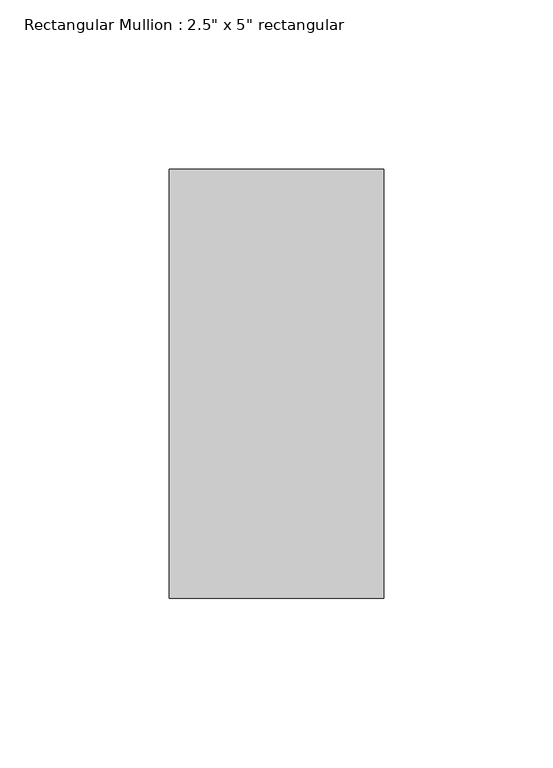
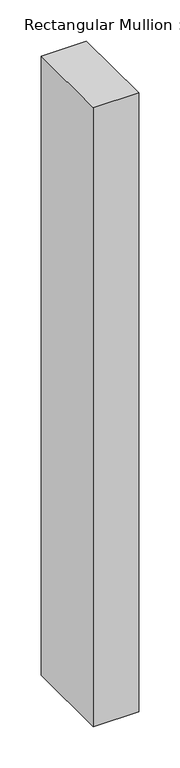
"""IFC4 building model written with IfcOpenShell, lengths in millimetres: member geometry."""

from ifc_helpers import new_model, si_unit, frame, origin, place, context, project, spatial, polyline, outline, extrude, source, transform, mapped, element, save


def member_54f829b7(model_context):
    return source(origin(), model_context, "Body", "SweptSolid", [
        extrude(outline(polyline([(31.75, 63.5), (31.75, -63.5), (-31.75, -63.5), (-31.75, 63.5), (31.75, 63.5)])), frame((0.0, 0.0, -918.7415583), z_axis=(0.0, 0.0, 1.0), x_axis=(1.0, 0.0, 0.0)), (0.0, 0.0, 1.0), 918.7415583),
    ])


if __name__ == "__main__":
    model = new_model("IFC4")
    model_context = context("Model", 3, world=origin())
    ifc_project = project(units=[si_unit("LENGTHUNIT", "METRE", prefix="MILLI")], contexts=[model_context])
    site = spatial("IfcSite", under=ifc_project)
    building = spatial("IfcBuilding", under=site)
    placement = place(None, origin())
    member_shape = member_54f829b7(model_context)
    element("IfcMember", 1, ObjectType="Rectangular Mullion : 2.5\" x 5\" rectangular", at=placement, inside=building, context=model_context, shape_type="MappedRepresentation", body=[
        mapped(member_shape, transform((0.0, 0.0, 0.0), x_axis=(1.0, 0.0, 0.0), y_axis=(0.0, 1.0, 0.0), z_axis=(0.0, 0.0, 1.0))),
    ])
    save(model, "model.ifc")

# Revit data of these elements
# Type "Rectangular Mullion : 2.5\" x 5\" rectangular"
#   built-in parameter 1007304 = 0.416667 (stored number, unit not read)
#   built-in parameter 1007301 = 0.104167 (stored number, unit not read)
#   built-in parameter 1007300 = 0.104167 (stored number, unit not read)
# Element 1 (IfcMember, "Rectangular Mullion : 2.5\" x 5\" rectangular")
#   Materials on its faces: "Aluminum"
# Materials
#   "Aluminum": class "Metal", colour RGB 247 247 247, transparency 0, Description = "Aluminum 6061", Cost = 0
